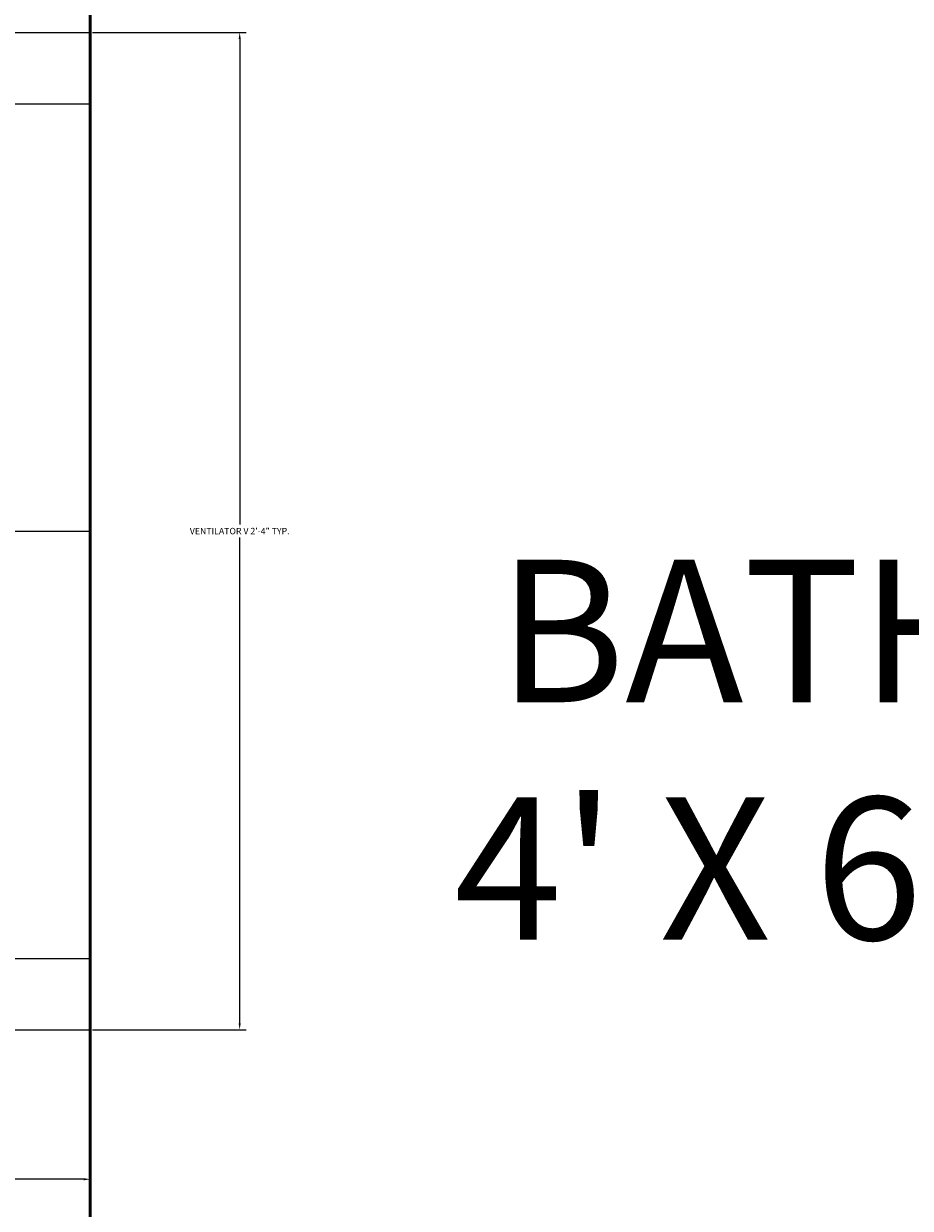
# Model space of a CAD drawing. Units: inches. Extents: x 37 to 824, y -700 to 234.
# Tile 45 of 77: x 168 to 193, y 17 to 50. Entities that reach past the tile are written whole.
import ezdxf

# ---------------------------------------------------------------- set-up
doc = ezdxf.new("R2010")
doc.units = ezdxf.units.IN
doc.header["$MEASUREMENT"] = 0
for name, color, linetype, lineweight in [('A-ANNO-DIMS', 2, 'Continuous', 18), ('A-AREA-IDEN', 3, 'Continuous', 18), ('A-GLAZ', 4, 'Continuous', 25), ('A-WALL', 2, 'Continuous', 50)]:
    doc.layers.add(name, color=color, linetype=linetype, lineweight=lineweight)
doc.styles.get("Standard").update_dxf_attribs({"font": 'arial.ttf'})
doc.dimstyles.get("Standard").update_dxf_attribs({"dimtxt": 0.18, "dimasz": 0.18, "dimexe": 0.18, "dimexo": 0.0625, "dimgap": 0.09, "dimtad": 0, "dimtih": 1, "dimtoh": 1, "dimdec": 1, "dimzin": 0, "dimdsep": 46, "dimlunit": 4, "dimtxsty": 'Standard', "dimcen": 0.09, "dimadec": 0, "dimazin": 0, "dimtfac": 1, "dimtdec": 1, "dimtofl": 0, "dimtmove": 0, "dimatfit": 3, "dimfxl": 1, "dimtolj": 1, "dimtzin": 0, "dimarcsym": 0})

# ---------------------------------------------------------------- blocks, each defined once
blk = doc.blocks.new('VENT-600')
for p, q in [((0, 28), (9, 28)), ((0, 26), (9, 26)), ((3.5, 26), (3.5, 2)), ((5.5, 26), (5.5, 2)), ((0, 14), (9, 14)), ((0, 2), (9, 2)), ((0, 0), (9, 0))]:
    blk.add_line(p, q)
blk = doc.blocks.new('*D40')
at = {"layer": 'A-ANNO-DIMS', "color": 0, "lineweight": -2, "ltscale": 0.5, "transparency": 16777216}
for p, q in [((170.14, 50.09), (174.457, 50.09)), ((174.277, 49.91), (174.277, 36.274)), ((174.277, 22.27), (174.277, 35.907)), ((170.14, 22.09), (174.457, 22.09))]:
    blk.add_line(p, q, dxfattribs=at)
at = {"layer": 'A-ANNO-DIMS', "color": 0, "ltscale": 0.5, "transparency": 16777216}
for points in [[(174.247, 49.91), (174.307, 49.91), (174.277, 50.09)], [(174.247, 22.27), (174.307, 22.27), (174.277, 22.09)]]:
    blk.add_solid(points, dxfattribs=at)
at = {"layer": 'Defpoints', "color": 0, "ltscale": 0.5, "transparency": 16777216}
for p in [(170.077, 50.09), (174.277, 50.09), (170.077, 22.09)]:
    blk.add_point(p, dxfattribs=at)
at = {"layer": 'A-ANNO-DIMS', "color": 0, "ltscale": 0.5, "transparency": 16777216, "insert": (174.277, 36.09), "char_height": 0.18, "attachment_point": 5}
blk.add_mtext('\\A1;VENTILATOR V 2\'-4" TYP.', dxfattribs=at)
blk = doc.blocks.new('*D41')
at = {"layer": 'A-ANNO-DIMS', "color": 0, "lineweight": -2, "ltscale": 0.5, "transparency": 16777216}
for p, q in [((161.077, 22.028), (161.077, 17.71)), ((170.077, 22.028), (170.077, 17.71)), ((161.257, 17.89), (164.939, 17.89)), ((169.897, 17.89), (166.216, 17.89))]:
    blk.add_line(p, q, dxfattribs=at)
at = {"layer": 'A-ANNO-DIMS', "color": 0, "ltscale": 0.5, "transparency": 16777216}
for points in [[(161.257, 17.92), (161.257, 17.86), (161.077, 17.89)], [(169.897, 17.92), (169.897, 17.86), (170.077, 17.89)]]:
    blk.add_solid(points, dxfattribs=at)
at = {"layer": 'Defpoints', "color": 0, "ltscale": 0.5, "transparency": 16777216}
for p in [(161.077, 22.09), (170.077, 22.09), (170.077, 17.89)]:
    blk.add_point(p, dxfattribs=at)
at = {"layer": 'A-ANNO-DIMS', "color": 0, "ltscale": 0.5, "transparency": 16777216, "insert": (165.577, 17.89), "char_height": 0.18, "attachment_point": 5}
blk.add_mtext('\\A1;0\'-9" TYP.', dxfattribs=at)
blk = doc.blocks.new('*D84')
at = {"layer": 'A-ANNO-DIMS', "color": 0, "lineweight": -2, "ltscale": 0.5, "transparency": 16777216}
for p, q in [((170.077, -265.847), (170.077, 234.17)), ((210.077, -265.847), (210.077, 234.17)), ((170.257, 233.99), (189.748, 233.99)), ((209.897, 233.99), (190.406, 233.99))]:
    blk.add_line(p, q, dxfattribs=at)
at = {"layer": 'A-ANNO-DIMS', "color": 0, "ltscale": 0.5, "transparency": 16777216}
for points in [[(170.257, 234.02), (170.257, 233.96), (170.077, 233.99)], [(209.897, 234.02), (209.897, 233.96), (210.077, 233.99)]]:
    blk.add_solid(points, dxfattribs=at)
at = {"layer": 'Defpoints', "color": 0, "ltscale": 0.5, "transparency": 16777216}
for p in [(210.077, 233.99), (170.077, -265.91), (210.077, -265.91)]:
    blk.add_point(p, dxfattribs=at)
at = {"layer": 'A-ANNO-DIMS', "color": 0, "ltscale": 0.5, "transparency": 16777216, "insert": (190.077, 233.99), "char_height": 0.18, "attachment_point": 5}
blk.add_mtext('\\A1;3\'-4"', dxfattribs=at)
blk = doc.blocks.new('*D85')
at = {"layer": 'A-ANNO-DIMS', "color": 0, "lineweight": -2, "ltscale": 0.5, "transparency": 16777216}
for p, q in [((170.077, -356.847), (170.077, 234.17)), ((206.077, -356.847), (206.077, 234.17)), ((170.257, 233.99), (187.748, 233.99)), ((205.897, 233.99), (188.406, 233.99))]:
    blk.add_line(p, q, dxfattribs=at)
at = {"layer": 'A-ANNO-DIMS', "color": 0, "ltscale": 0.5, "transparency": 16777216}
for points in [[(170.257, 234.02), (170.257, 233.96), (170.077, 233.99)], [(205.897, 234.02), (205.897, 233.96), (206.077, 233.99)]]:
    blk.add_solid(points, dxfattribs=at)
at = {"layer": 'Defpoints', "color": 0, "ltscale": 0.5, "transparency": 16777216}
for p in [(206.077, 233.99), (170.077, -356.91), (206.077, -356.91)]:
    blk.add_point(p, dxfattribs=at)
at = {"layer": 'A-ANNO-DIMS', "color": 0, "ltscale": 0.5, "transparency": 16777216, "insert": (188.077, 233.99), "char_height": 0.18, "attachment_point": 5}
blk.add_mtext('\\A1;3\'-0"', dxfattribs=at)

msp = doc.modelspace()

# ---------------------------------------------------------------- linework, layer by layer
at = {"layer": 'A-WALL'}
msp.add_line((170.077, 75.09), (170.077, -2.91), dxfattribs=at)

# ---------------------------------------------------------------- block references
at = {"layer": 'A-GLAZ'}
msp.add_blockref('VENT-600', (161.077, 22.09), dxfattribs=at)

# ---------------------------------------------------------------- texts
at = {"layer": 'A-AREA-IDEN', "insert": (176.627, 35.284), "char_height": 4, "attachment_point": 1}
msp.add_mtext_dynamic_manual_height_columns('    BATH\\P   4\' X 6\'6"', width=88.32168, gutter_width=1, heights=[0], dxfattribs=at)

# ---------------------------------------------------------------- dimensions: what is measured, and where the dimension line sits
at = {"layer": 'A-ANNO-DIMS', "ltscale": 0.5}
for base, p1, p2, picture, middle in [((210.077, 233.99), (170.077, -265.91), (210.077, -265.91), '*D84', (190.077, 233.99)), ((206.077, 233.99), (170.077, -356.91), (206.077, -356.91), '*D85', (188.077, 233.99))]:
    dim = msp.add_linear_dim(base=base, p1=p1, p2=p2, dimstyle='Standard', override={"dimdec": 1, "dimlfac": 1, "dimrnd": 0, "dimzin": 1, "dimdsep": 46, "dimlunit": 4, "dimfrac": 2}, dxfattribs=at)
    dim.commit()
    dim.dimension.update_dxf_attribs({"geometry": picture, "text_midpoint": middle})
dim = msp.add_linear_dim(base=(174.277, 50.09), p1=(170.077, 22.09), p2=(170.077, 50.09), angle=90, text='VENTILATOR V <> TYP.', dimstyle='Standard', override={"dimdec": 1, "dimlfac": 1, "dimrnd": 0, "dimzin": 1, "dimdsep": 46, "dimlunit": 4, "dimfrac": 2}, dxfattribs=at)
dim.commit()
dim.dimension.update_dxf_attribs({"geometry": '*D40', "text_midpoint": (174.277, 36.09)})
dim = msp.add_linear_dim(base=(170.077, 17.89), p1=(161.077, 22.09), p2=(170.077, 22.09), text='<> TYP.', dimstyle='Standard', override={"dimdec": 1, "dimlfac": 1, "dimrnd": 0, "dimzin": 1, "dimdsep": 46, "dimlunit": 4, "dimfrac": 2}, dxfattribs=at)
dim.commit()
dim.dimension.update_dxf_attribs({"geometry": '*D41', "text_midpoint": (165.577, 17.89)})

doc.saveas('drawing.dxf')
